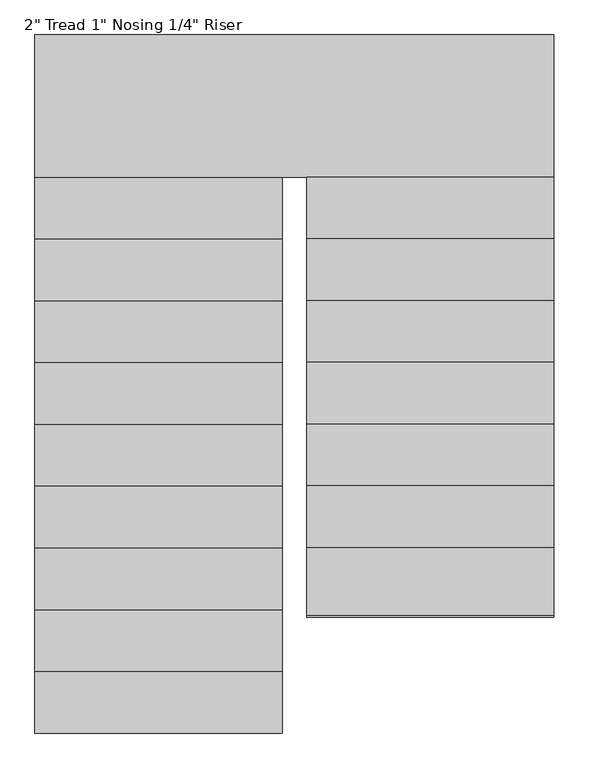
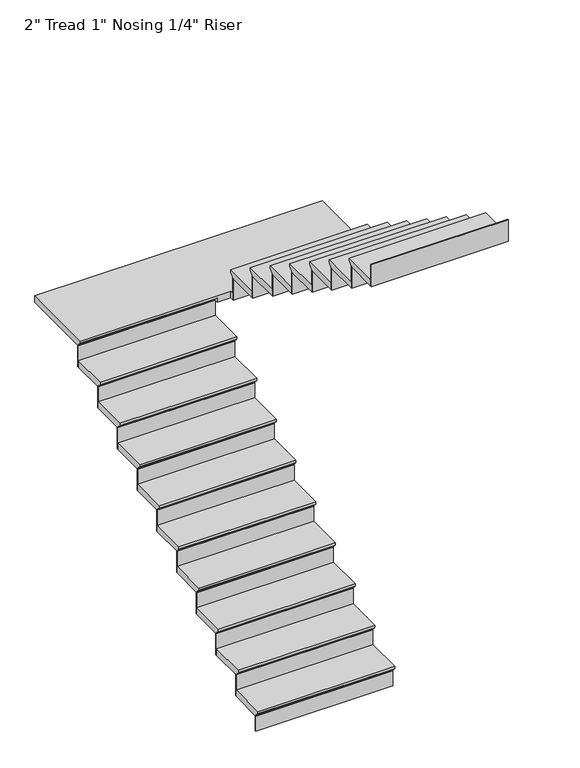
"""IFC4 building model written with IfcOpenShell, lengths in millimetres: stair flight geometry."""

from ifc_helpers import new_model, si_unit, origin, place, context, project, spatial, faceted_brep, source, transform, mapped, element, save


def stair_flight_95751e6d(model_context):
    return source(origin(), model_context, "Body", "Brep", [
        faceted_brep([(-8657.8672301, -3404.4302427, 455.0833333), (-8657.8672301, -3404.4302427, 474.1333333), (-9673.8672301, -3404.4302427, 474.1333333), (-9673.8672301, -3404.4302427, 455.0833333), (-8657.8672301, -3379.0302427, 429.6833333), (-9673.8672301, -3379.0302427, 429.6833333), (-8657.8672301, -3125.0302427, 474.1333333), (-9673.8672301, -3125.0302427, 474.1333333), (-9673.8672301, -3379.0302427, 423.3333333), (-9673.8672301, -3125.0302427, 423.3333333), (-8657.8672301, -3125.0302427, 423.3333333), (-8657.8672301, -3379.0302427, 423.3333333)], [[[0, 1, 2, 3]], [[4, 0, 3, 5]], [[2, 1, 6, 7]], [[8, 9, 10, 11]], [[2, 7, 9, 8, 5, 3]], [[8, 11, 4, 5]], [[6, 1, 0, 4, 11, 10]], [[7, 6, 10, 9]]]),
        faceted_brep([(-8657.8672301, -3379.0302427, 423.3333333), (-8657.8672301, -3379.0302427, 304.8), (-8657.8672301, -3372.6802427, 304.8), (-8657.8672301, -3372.6802427, 423.3333333), (-9673.8672301, -3379.0302427, 423.3333333), (-9673.8672301, -3372.6802427, 423.3333333), (-9673.8672301, -3372.6802427, 304.8), (-9673.8672301, -3379.0302427, 304.8)], [[[0, 1, 2, 3]], [[4, 5, 6, 7]], [[1, 0, 4, 7]], [[2, 1, 7, 6]], [[3, 2, 6, 5]], [[0, 3, 5, 4]]]),
        faceted_brep([(-8657.8672301, -3125.0302427, 592.6666667), (-8657.8672301, -3125.0302427, 423.3333333), (-8657.8672301, -3118.6802427, 423.3333333), (-8657.8672301, -3118.6802427, 592.6666667), (-9673.8672301, -3125.0302427, 592.6666667), (-9673.8672301, -3118.6802427, 592.6666667), (-9673.8672301, -3118.6802427, 423.3333333), (-9673.8672301, -3125.0302427, 423.3333333)], [[[0, 1, 2, 3]], [[4, 5, 6, 7]], [[1, 0, 4, 7]], [[2, 1, 7, 6]], [[3, 2, 6, 5]], [[0, 3, 5, 4]]]),
        faceted_brep([(-9673.8672301, -3150.4302427, 643.4666667), (-8657.8672301, -3150.4302427, 643.4666667), (-8657.8672301, -2871.0302427, 643.4666667), (-9673.8672301, -2871.0302427, 643.4666667), (-9673.8672301, -3125.0302427, 592.6666667), (-9673.8672301, -2871.0302427, 592.6666667), (-8657.8672301, -2871.0302427, 592.6666667), (-8657.8672301, -3125.0302427, 592.6666667), (-9673.8672301, -3125.0302427, 599.0166667), (-9673.8672301, -3150.4302427, 624.4166667), (-8657.8672301, -3125.0302427, 599.0166667), (-8657.8672301, -3150.4302427, 624.4166667)], [[[0, 1, 2, 3]], [[4, 5, 6, 7]], [[0, 3, 5, 4, 8, 9]], [[4, 7, 10, 8]], [[2, 1, 11, 10, 7, 6]], [[3, 2, 6, 5]], [[11, 1, 0, 9]], [[10, 11, 9, 8]]]),
        faceted_brep([(-8657.8672301, -2871.0302427, 762.0), (-8657.8672301, -2871.0302427, 592.6666667), (-8657.8672301, -2864.6802427, 592.6666667), (-8657.8672301, -2864.6802427, 762.0), (-9673.8672301, -2871.0302427, 762.0), (-9673.8672301, -2864.6802427, 762.0), (-9673.8672301, -2864.6802427, 592.6666667), (-9673.8672301, -2871.0302427, 592.6666667)], [[[0, 1, 2, 3]], [[4, 5, 6, 7]], [[1, 0, 4, 7]], [[2, 1, 7, 6]], [[3, 2, 6, 5]], [[0, 3, 5, 4]]]),
        faceted_brep([(-9673.8672301, -2896.4302427, 812.8), (-8657.8672301, -2896.4302427, 812.8), (-8657.8672301, -2617.0302427, 812.8), (-9673.8672301, -2617.0302427, 812.8), (-9673.8672301, -2871.0302427, 762.0), (-9673.8672301, -2617.0302427, 762.0), (-8657.8672301, -2617.0302427, 762.0), (-8657.8672301, -2871.0302427, 762.0), (-9673.8672301, -2871.0302427, 768.35), (-9673.8672301, -2896.4302427, 793.75), (-8657.8672301, -2871.0302427, 768.35), (-8657.8672301, -2896.4302427, 793.75)], [[[0, 1, 2, 3]], [[4, 5, 6, 7]], [[0, 3, 5, 4, 8, 9]], [[4, 7, 10, 8]], [[2, 1, 11, 10, 7, 6]], [[3, 2, 6, 5]], [[11, 1, 0, 9]], [[10, 11, 9, 8]]]),
        faceted_brep([(-8657.8672301, -2617.0302427, 931.3333333), (-8657.8672301, -2617.0302427, 762.0), (-8657.8672301, -2610.6802427, 762.0), (-8657.8672301, -2610.6802427, 931.3333333), (-9673.8672301, -2617.0302427, 931.3333333), (-9673.8672301, -2610.6802427, 931.3333333), (-9673.8672301, -2610.6802427, 762.0), (-9673.8672301, -2617.0302427, 762.0)], [[[0, 1, 2, 3]], [[4, 5, 6, 7]], [[1, 0, 4, 7]], [[2, 1, 7, 6]], [[3, 2, 6, 5]], [[0, 3, 5, 4]]]),
        faceted_brep([(-9673.8672301, -2642.4302427, 982.1333333), (-8657.8672301, -2642.4302427, 982.1333333), (-8657.8672301, -2363.0302427, 982.1333333), (-9673.8672301, -2363.0302427, 982.1333333), (-9673.8672301, -2617.0302427, 931.3333333), (-9673.8672301, -2363.0302427, 931.3333333), (-8657.8672301, -2363.0302427, 931.3333333), (-8657.8672301, -2617.0302427, 931.3333333), (-9673.8672301, -2617.0302427, 937.6833333), (-9673.8672301, -2642.4302427, 963.0833333), (-8657.8672301, -2617.0302427, 937.6833333), (-8657.8672301, -2642.4302427, 963.0833333)], [[[0, 1, 2, 3]], [[4, 5, 6, 7]], [[0, 3, 5, 4, 8, 9]], [[4, 7, 10, 8]], [[2, 1, 11, 10, 7, 6]], [[3, 2, 6, 5]], [[11, 1, 0, 9]], [[10, 11, 9, 8]]]),
        faceted_brep([(-8657.8672301, -2363.0302427, 1100.6666667), (-8657.8672301, -2363.0302427, 931.3333333), (-8657.8672301, -2356.6802427, 931.3333333), (-8657.8672301, -2356.6802427, 1100.6666667), (-9673.8672301, -2363.0302427, 1100.6666667), (-9673.8672301, -2356.6802427, 1100.6666667), (-9673.8672301, -2356.6802427, 931.3333333), (-9673.8672301, -2363.0302427, 931.3333333)], [[[0, 1, 2, 3]], [[4, 5, 6, 7]], [[1, 0, 4, 7]], [[2, 1, 7, 6]], [[3, 2, 6, 5]], [[0, 3, 5, 4]]]),
        faceted_brep([(-9673.8672301, -2388.4302427, 1151.4666667), (-8657.8672301, -2388.4302427, 1151.4666667), (-8657.8672301, -2109.0302427, 1151.4666667), (-9673.8672301, -2109.0302427, 1151.4666667), (-9673.8672301, -2363.0302427, 1100.6666667), (-9673.8672301, -2109.0302427, 1100.6666667), (-8657.8672301, -2109.0302427, 1100.6666667), (-8657.8672301, -2363.0302427, 1100.6666667), (-9673.8672301, -2363.0302427, 1107.0166667), (-9673.8672301, -2388.4302427, 1132.4166667), (-8657.8672301, -2363.0302427, 1107.0166667), (-8657.8672301, -2388.4302427, 1132.4166667)], [[[0, 1, 2, 3]], [[4, 5, 6, 7]], [[0, 3, 5, 4, 8, 9]], [[4, 7, 10, 8]], [[2, 1, 11, 10, 7, 6]], [[3, 2, 6, 5]], [[11, 1, 0, 9]], [[10, 11, 9, 8]]]),
        faceted_brep([(-8657.8672301, -2109.0302427, 1270.0), (-8657.8672301, -2109.0302427, 1100.6666667), (-8657.8672301, -2102.6802427, 1100.6666667), (-8657.8672301, -2102.6802427, 1270.0), (-9673.8672301, -2109.0302427, 1270.0), (-9673.8672301, -2102.6802427, 1270.0), (-9673.8672301, -2102.6802427, 1100.6666667), (-9673.8672301, -2109.0302427, 1100.6666667)], [[[0, 1, 2, 3]], [[4, 5, 6, 7]], [[1, 0, 4, 7]], [[2, 1, 7, 6]], [[3, 2, 6, 5]], [[0, 3, 5, 4]]]),
        faceted_brep([(-9673.8672301, -2134.4302427, 1320.8), (-8657.8672301, -2134.4302427, 1320.8), (-8657.8672301, -1855.0302427, 1320.8), (-9673.8672301, -1855.0302427, 1320.8), (-9673.8672301, -2109.0302427, 1270.0), (-9673.8672301, -1855.0302427, 1270.0), (-8657.8672301, -1855.0302427, 1270.0), (-8657.8672301, -2109.0302427, 1270.0), (-9673.8672301, -2109.0302427, 1276.35), (-9673.8672301, -2134.4302427, 1301.75), (-8657.8672301, -2109.0302427, 1276.35), (-8657.8672301, -2134.4302427, 1301.75)], [[[0, 1, 2, 3]], [[4, 5, 6, 7]], [[0, 3, 5, 4, 8, 9]], [[4, 7, 10, 8]], [[2, 1, 11, 10, 7, 6]], [[3, 2, 6, 5]], [[11, 1, 0, 9]], [[10, 11, 9, 8]]]),
        faceted_brep([(-8657.8672301, -1855.0302427, 1439.3333333), (-8657.8672301, -1855.0302427, 1270.0), (-8657.8672301, -1848.6802427, 1270.0), (-8657.8672301, -1848.6802427, 1439.3333333), (-9673.8672301, -1855.0302427, 1439.3333333), (-9673.8672301, -1848.6802427, 1439.3333333), (-9673.8672301, -1848.6802427, 1270.0), (-9673.8672301, -1855.0302427, 1270.0)], [[[0, 1, 2, 3]], [[4, 5, 6, 7]], [[1, 0, 4, 7]], [[2, 1, 7, 6]], [[3, 2, 6, 5]], [[0, 3, 5, 4]]]),
        faceted_brep([(-9673.8672301, -1880.4302427, 1490.1333333), (-8657.8672301, -1880.4302427, 1490.1333333), (-8657.8672301, -1601.0302427, 1490.1333333), (-9673.8672301, -1601.0302427, 1490.1333333), (-9673.8672301, -1855.0302427, 1439.3333333), (-9673.8672301, -1601.0302427, 1439.3333333), (-8657.8672301, -1601.0302427, 1439.3333333), (-8657.8672301, -1855.0302427, 1439.3333333), (-9673.8672301, -1855.0302427, 1445.6833333), (-9673.8672301, -1880.4302427, 1471.0833333), (-8657.8672301, -1855.0302427, 1445.6833333), (-8657.8672301, -1880.4302427, 1471.0833333)], [[[0, 1, 2, 3]], [[4, 5, 6, 7]], [[0, 3, 5, 4, 8, 9]], [[4, 7, 10, 8]], [[2, 1, 11, 10, 7, 6]], [[3, 2, 6, 5]], [[11, 1, 0, 9]], [[10, 11, 9, 8]]]),
        faceted_brep([(-8657.8672301, -1601.0302427, 1608.6666667), (-8657.8672301, -1601.0302427, 1439.3333333), (-8657.8672301, -1594.6802427, 1439.3333333), (-8657.8672301, -1594.6802427, 1608.6666667), (-9673.8672301, -1601.0302427, 1608.6666667), (-9673.8672301, -1594.6802427, 1608.6666667), (-9673.8672301, -1594.6802427, 1439.3333333), (-9673.8672301, -1601.0302427, 1439.3333333)], [[[0, 1, 2, 3]], [[4, 5, 6, 7]], [[1, 0, 4, 7]], [[2, 1, 7, 6]], [[3, 2, 6, 5]], [[0, 3, 5, 4]]]),
        faceted_brep([(-9673.8672301, -1626.4302427, 1659.4666667), (-8657.8672301, -1626.4302427, 1659.4666667), (-8657.8672301, -1347.0302427, 1659.4666667), (-9673.8672301, -1347.0302427, 1659.4666667), (-9673.8672301, -1601.0302427, 1608.6666667), (-9673.8672301, -1347.0302427, 1608.6666667), (-8657.8672301, -1347.0302427, 1608.6666667), (-8657.8672301, -1601.0302427, 1608.6666667), (-9673.8672301, -1601.0302427, 1615.0166667), (-9673.8672301, -1626.4302427, 1640.4166667), (-8657.8672301, -1601.0302427, 1615.0166667), (-8657.8672301, -1626.4302427, 1640.4166667)], [[[0, 1, 2, 3]], [[4, 5, 6, 7]], [[0, 3, 5, 4, 8, 9]], [[4, 7, 10, 8]], [[2, 1, 11, 10, 7, 6]], [[3, 2, 6, 5]], [[11, 1, 0, 9]], [[10, 11, 9, 8]]]),
        faceted_brep([(-8657.8672301, -1347.0302427, 1778.0), (-8657.8672301, -1347.0302427, 1608.6666667), (-8657.8672301, -1340.6802427, 1608.6666667), (-8657.8672301, -1340.6802427, 1778.0), (-9673.8672301, -1347.0302427, 1778.0), (-9673.8672301, -1340.6802427, 1778.0), (-9673.8672301, -1340.6802427, 1608.6666667), (-9673.8672301, -1347.0302427, 1608.6666667)], [[[0, 1, 2, 3]], [[4, 5, 6, 7]], [[1, 0, 4, 7]], [[2, 1, 7, 6]], [[3, 2, 6, 5]], [[0, 3, 5, 4]]]),
        faceted_brep([(-9673.8672301, -1372.4302427, 1828.8), (-8657.8672301, -1372.4302427, 1828.8), (-8657.8672301, -1093.0302427, 1828.8), (-9673.8672301, -1093.0302427, 1828.8), (-9673.8672301, -1347.0302427, 1778.0), (-9673.8672301, -1093.0302427, 1778.0), (-8657.8672301, -1093.0302427, 1778.0), (-8657.8672301, -1347.0302427, 1778.0), (-9673.8672301, -1347.0302427, 1784.35), (-9673.8672301, -1372.4302427, 1809.75), (-8657.8672301, -1347.0302427, 1784.35), (-8657.8672301, -1372.4302427, 1809.75)], [[[0, 1, 2, 3]], [[4, 5, 6, 7]], [[0, 3, 5, 4, 8, 9]], [[4, 7, 10, 8]], [[2, 1, 11, 10, 7, 6]], [[3, 2, 6, 5]], [[11, 1, 0, 9]], [[10, 11, 9, 8]]]),
        faceted_brep([(-8657.8672301, -1093.0302427, 1947.3333333), (-8657.8672301, -1093.0302427, 1778.0), (-8657.8672301, -1086.6802427, 1778.0), (-8657.8672301, -1086.6802427, 1947.3333333), (-9673.8672301, -1093.0302427, 1947.3333333), (-9673.8672301, -1086.6802427, 1947.3333333), (-9673.8672301, -1086.6802427, 1778.0), (-9673.8672301, -1093.0302427, 1778.0)], [[[0, 1, 2, 3]], [[4, 5, 6, 7]], [[1, 0, 4, 7]], [[2, 1, 7, 6]], [[3, 2, 6, 5]], [[0, 3, 5, 4]]]),
        faceted_brep([(-7540.2672301, -1143.8302427, 1998.1333333), (-7540.2672301, -534.2302427, 1998.1333333), (-9673.8672301, -534.2302427, 1998.1333333), (-9673.8672301, -1118.4302427, 1998.1333333), (-8556.2672301, -1118.4302427, 1998.1333333), (-8556.2672301, -1143.8302427, 1998.1333333), (-7540.2672301, -534.2302427, 1947.3333333), (-7540.2672301, -1143.8302427, 1947.3333333), (-8556.2672301, -1143.8302427, 1947.3333333), (-8556.2672301, -1118.4302427, 1947.3333333), (-8657.8672301, -1118.4302427, 1947.3333333), (-8657.8672301, -1093.0302427, 1947.3333333), (-9673.8672301, -1093.0302427, 1947.3333333), (-9673.8672301, -534.2302427, 1947.3333333), (-9673.8672301, -1093.0302427, 1953.6833333), (-9673.8672301, -1118.4302427, 1979.0833333), (-8657.8672301, -1093.0302427, 1953.6833333), (-8657.8672301, -1118.4302427, 1979.0833333)], [[[0, 1, 2, 3, 4, 5]], [[6, 7, 8, 9, 10, 11, 12, 13]], [[1, 0, 7, 6]], [[2, 1, 6, 13]], [[3, 2, 13, 12, 14, 15]], [[12, 11, 16, 14]], [[11, 10, 17, 16]], [[4, 3, 15, 17, 10, 9]], [[5, 4, 9, 8]], [[0, 5, 8, 7]], [[15, 14, 16, 17]]]),
        faceted_brep([(-8556.2672301, -1143.8302427, 2116.6666667), (-8556.2672301, -1143.8302427, 1947.3333333), (-8556.2672301, -1150.1802427, 1947.3333333), (-8556.2672301, -1150.1802427, 2116.6666667), (-7540.2672301, -1143.8302427, 2116.6666667), (-7540.2672301, -1150.1802427, 2116.6666667), (-7540.2672301, -1150.1802427, 1947.3333333), (-7540.2672301, -1143.8302427, 1947.3333333)], [[[0, 1, 2, 3]], [[4, 5, 6, 7]], [[1, 0, 4, 7]], [[2, 1, 7, 6]], [[3, 2, 6, 5]], [[0, 3, 5, 4]]]),
        faceted_brep([(-7540.2672301, -1118.4302427, 2167.4666667), (-8556.2672301, -1118.4302427, 2167.4666667), (-8556.2672301, -1397.8302427, 2167.4666667), (-7540.2672301, -1397.8302427, 2167.4666667), (-7540.2672301, -1143.8302427, 2116.6666667), (-7540.2672301, -1397.8302427, 2116.6666667), (-8556.2672301, -1397.8302427, 2116.6666667), (-8556.2672301, -1143.8302427, 2116.6666667), (-7540.2672301, -1143.8302427, 2123.0166667), (-7540.2672301, -1118.4302427, 2148.4166667), (-8556.2672301, -1143.8302427, 2123.0166667), (-8556.2672301, -1118.4302427, 2148.4166667)], [[[0, 1, 2, 3]], [[4, 5, 6, 7]], [[0, 3, 5, 4, 8, 9]], [[4, 7, 10, 8]], [[2, 1, 11, 10, 7, 6]], [[3, 2, 6, 5]], [[11, 1, 0, 9]], [[10, 11, 9, 8]]]),
        faceted_brep([(-8556.2672301, -1397.8302427, 2286.0), (-8556.2672301, -1397.8302427, 2116.6666667), (-8556.2672301, -1404.1802427, 2116.6666667), (-8556.2672301, -1404.1802427, 2286.0), (-7540.2672301, -1397.8302427, 2286.0), (-7540.2672301, -1404.1802427, 2286.0), (-7540.2672301, -1404.1802427, 2116.6666667), (-7540.2672301, -1397.8302427, 2116.6666667)], [[[0, 1, 2, 3]], [[4, 5, 6, 7]], [[1, 0, 4, 7]], [[2, 1, 7, 6]], [[3, 2, 6, 5]], [[0, 3, 5, 4]]]),
        faceted_brep([(-7540.2672301, -1372.4302427, 2336.8), (-8556.2672301, -1372.4302427, 2336.8), (-8556.2672301, -1651.8302427, 2336.8), (-7540.2672301, -1651.8302427, 2336.8), (-7540.2672301, -1397.8302427, 2286.0), (-7540.2672301, -1651.8302427, 2286.0), (-8556.2672301, -1651.8302427, 2286.0), (-8556.2672301, -1397.8302427, 2286.0), (-7540.2672301, -1397.8302427, 2292.35), (-7540.2672301, -1372.4302427, 2317.75), (-8556.2672301, -1397.8302427, 2292.35), (-8556.2672301, -1372.4302427, 2317.75)], [[[0, 1, 2, 3]], [[4, 5, 6, 7]], [[0, 3, 5, 4, 8, 9]], [[4, 7, 10, 8]], [[2, 1, 11, 10, 7, 6]], [[3, 2, 6, 5]], [[11, 1, 0, 9]], [[10, 11, 9, 8]]]),
        faceted_brep([(-8556.2672301, -1651.8302427, 2455.3333333), (-8556.2672301, -1651.8302427, 2286.0), (-8556.2672301, -1658.1802427, 2286.0), (-8556.2672301, -1658.1802427, 2455.3333333), (-7540.2672301, -1651.8302427, 2455.3333333), (-7540.2672301, -1658.1802427, 2455.3333333), (-7540.2672301, -1658.1802427, 2286.0), (-7540.2672301, -1651.8302427, 2286.0)], [[[0, 1, 2, 3]], [[4, 5, 6, 7]], [[1, 0, 4, 7]], [[2, 1, 7, 6]], [[3, 2, 6, 5]], [[0, 3, 5, 4]]]),
        faceted_brep([(-7540.2672301, -1626.4302427, 2506.1333333), (-8556.2672301, -1626.4302427, 2506.1333333), (-8556.2672301, -1905.8302427, 2506.1333333), (-7540.2672301, -1905.8302427, 2506.1333333), (-7540.2672301, -1651.8302427, 2455.3333333), (-7540.2672301, -1905.8302427, 2455.3333333), (-8556.2672301, -1905.8302427, 2455.3333333), (-8556.2672301, -1651.8302427, 2455.3333333), (-7540.2672301, -1651.8302427, 2461.6833333), (-7540.2672301, -1626.4302427, 2487.0833333), (-8556.2672301, -1651.8302427, 2461.6833333), (-8556.2672301, -1626.4302427, 2487.0833333)], [[[0, 1, 2, 3]], [[4, 5, 6, 7]], [[0, 3, 5, 4, 8, 9]], [[4, 7, 10, 8]], [[2, 1, 11, 10, 7, 6]], [[3, 2, 6, 5]], [[11, 1, 0, 9]], [[10, 11, 9, 8]]]),
        faceted_brep([(-8556.2672301, -1905.8302427, 2624.6666667), (-8556.2672301, -1905.8302427, 2455.3333333), (-8556.2672301, -1912.1802427, 2455.3333333), (-8556.2672301, -1912.1802427, 2624.6666667), (-7540.2672301, -1905.8302427, 2624.6666667), (-7540.2672301, -1912.1802427, 2624.6666667), (-7540.2672301, -1912.1802427, 2455.3333333), (-7540.2672301, -1905.8302427, 2455.3333333)], [[[0, 1, 2, 3]], [[4, 5, 6, 7]], [[1, 0, 4, 7]], [[2, 1, 7, 6]], [[3, 2, 6, 5]], [[0, 3, 5, 4]]]),
        faceted_brep([(-7540.2672301, -1880.4302427, 2675.4666667), (-8556.2672301, -1880.4302427, 2675.4666667), (-8556.2672301, -2159.8302427, 2675.4666667), (-7540.2672301, -2159.8302427, 2675.4666667), (-7540.2672301, -1905.8302427, 2624.6666667), (-7540.2672301, -2159.8302427, 2624.6666667), (-8556.2672301, -2159.8302427, 2624.6666667), (-8556.2672301, -1905.8302427, 2624.6666667), (-7540.2672301, -1905.8302427, 2631.0166667), (-7540.2672301, -1880.4302427, 2656.4166667), (-8556.2672301, -1905.8302427, 2631.0166667), (-8556.2672301, -1880.4302427, 2656.4166667)], [[[0, 1, 2, 3]], [[4, 5, 6, 7]], [[0, 3, 5, 4, 8, 9]], [[4, 7, 10, 8]], [[2, 1, 11, 10, 7, 6]], [[3, 2, 6, 5]], [[11, 1, 0, 9]], [[10, 11, 9, 8]]]),
        faceted_brep([(-8556.2672301, -2159.8302427, 2794.0), (-8556.2672301, -2159.8302427, 2624.6666667), (-8556.2672301, -2166.1802427, 2624.6666667), (-8556.2672301, -2166.1802427, 2794.0), (-7540.2672301, -2159.8302427, 2794.0), (-7540.2672301, -2166.1802427, 2794.0), (-7540.2672301, -2166.1802427, 2624.6666667), (-7540.2672301, -2159.8302427, 2624.6666667)], [[[0, 1, 2, 3]], [[4, 5, 6, 7]], [[1, 0, 4, 7]], [[2, 1, 7, 6]], [[3, 2, 6, 5]], [[0, 3, 5, 4]]]),
        faceted_brep([(-7540.2672301, -2134.4302427, 2844.8), (-8556.2672301, -2134.4302427, 2844.8), (-8556.2672301, -2413.8302427, 2844.8), (-7540.2672301, -2413.8302427, 2844.8), (-7540.2672301, -2159.8302427, 2794.0), (-7540.2672301, -2413.8302427, 2794.0), (-8556.2672301, -2413.8302427, 2794.0), (-8556.2672301, -2159.8302427, 2794.0), (-7540.2672301, -2159.8302427, 2800.35), (-7540.2672301, -2134.4302427, 2825.75), (-8556.2672301, -2159.8302427, 2800.35), (-8556.2672301, -2134.4302427, 2825.75)], [[[0, 1, 2, 3]], [[4, 5, 6, 7]], [[0, 3, 5, 4, 8, 9]], [[4, 7, 10, 8]], [[2, 1, 11, 10, 7, 6]], [[3, 2, 6, 5]], [[11, 1, 0, 9]], [[10, 11, 9, 8]]]),
        faceted_brep([(-8556.2672301, -2413.8302427, 2963.3333333), (-8556.2672301, -2413.8302427, 2794.0), (-8556.2672301, -2420.1802427, 2794.0), (-8556.2672301, -2420.1802427, 2963.3333333), (-7540.2672301, -2413.8302427, 2963.3333333), (-7540.2672301, -2420.1802427, 2963.3333333), (-7540.2672301, -2420.1802427, 2794.0), (-7540.2672301, -2413.8302427, 2794.0)], [[[0, 1, 2, 3]], [[4, 5, 6, 7]], [[1, 0, 4, 7]], [[2, 1, 7, 6]], [[3, 2, 6, 5]], [[0, 3, 5, 4]]]),
        faceted_brep([(-7540.2672301, -2388.4302427, 3014.1333333), (-8556.2672301, -2388.4302427, 3014.1333333), (-8556.2672301, -2667.8302427, 3014.1333333), (-7540.2672301, -2667.8302427, 3014.1333333), (-7540.2672301, -2413.8302427, 2963.3333333), (-7540.2672301, -2667.8302427, 2963.3333333), (-8556.2672301, -2667.8302427, 2963.3333333), (-8556.2672301, -2413.8302427, 2963.3333333), (-7540.2672301, -2413.8302427, 2969.6833333), (-7540.2672301, -2388.4302427, 2995.0833333), (-8556.2672301, -2413.8302427, 2969.6833333), (-8556.2672301, -2388.4302427, 2995.0833333)], [[[0, 1, 2, 3]], [[4, 5, 6, 7]], [[0, 3, 5, 4, 8, 9]], [[4, 7, 10, 8]], [[2, 1, 11, 10, 7, 6]], [[3, 2, 6, 5]], [[11, 1, 0, 9]], [[10, 11, 9, 8]]]),
        faceted_brep([(-8556.2672301, -2667.8302427, 3132.6666667), (-8556.2672301, -2667.8302427, 2963.3333333), (-8556.2672301, -2674.1802427, 2963.3333333), (-8556.2672301, -2674.1802427, 3132.6666667), (-7540.2672301, -2667.8302427, 3132.6666667), (-7540.2672301, -2674.1802427, 3132.6666667), (-7540.2672301, -2674.1802427, 2963.3333333), (-7540.2672301, -2667.8302427, 2963.3333333)], [[[0, 1, 2, 3]], [[4, 5, 6, 7]], [[1, 0, 4, 7]], [[2, 1, 7, 6]], [[3, 2, 6, 5]], [[0, 3, 5, 4]]]),
        faceted_brep([(-8556.2672301, -2921.8302427, 3302.0), (-8556.2672301, -2921.8302427, 3132.6666667), (-8556.2672301, -2928.1802427, 3132.6666667), (-8556.2672301, -2928.1802427, 3302.0), (-7540.2672301, -2921.8302427, 3302.0), (-7540.2672301, -2928.1802427, 3302.0), (-7540.2672301, -2928.1802427, 3132.6666667), (-7540.2672301, -2921.8302427, 3132.6666667)], [[[0, 1, 2, 3]], [[4, 5, 6, 7]], [[1, 0, 4, 7]], [[2, 1, 7, 6]], [[3, 2, 6, 5]], [[0, 3, 5, 4]]]),
        faceted_brep([(-7540.2672301, -2642.4302427, 3183.4666667), (-8556.2672301, -2642.4302427, 3183.4666667), (-8556.2672301, -2921.8302427, 3183.4666667), (-7540.2672301, -2921.8302427, 3183.4666667), (-7540.2672301, -2667.8302427, 3132.6666667), (-7540.2672301, -2921.8302427, 3132.6666667), (-8556.2672301, -2921.8302427, 3132.6666667), (-8556.2672301, -2667.8302427, 3132.6666667), (-7540.2672301, -2667.8302427, 3139.0166667), (-7540.2672301, -2642.4302427, 3164.4166667), (-8556.2672301, -2667.8302427, 3139.0166667), (-8556.2672301, -2642.4302427, 3164.4166667)], [[[0, 1, 2, 3]], [[4, 5, 6, 7]], [[0, 3, 5, 4, 8, 9]], [[4, 7, 10, 8]], [[2, 1, 11, 10, 7, 6]], [[3, 2, 6, 5]], [[11, 1, 0, 9]], [[10, 11, 9, 8]]]),
    ])


if __name__ == "__main__":
    model = new_model("IFC4")
    model_context = context("Model", 3, world=origin())
    ifc_project = project(units=[si_unit("LENGTHUNIT", "METRE", prefix="MILLI")], contexts=[model_context])
    site = spatial("IfcSite", under=ifc_project)
    building = spatial("IfcBuilding", under=site)
    placement = place(None, origin())
    stair_flight_shape = stair_flight_95751e6d(model_context)
    element("IfcStairFlight", 1, ObjectType="2\" Tread 1\" Nosing 1/4\" Riser", at=placement, inside=building, context=model_context, shape_type="MappedRepresentation", body=[
        mapped(stair_flight_shape, transform((0.0, 0.0, 0.0), x_axis=(1.0, 0.0, 0.0), y_axis=(0.0, 1.0, 0.0), z_axis=(0.0, 0.0, 1.0))),
    ])
    save(model, "model.ifc")
